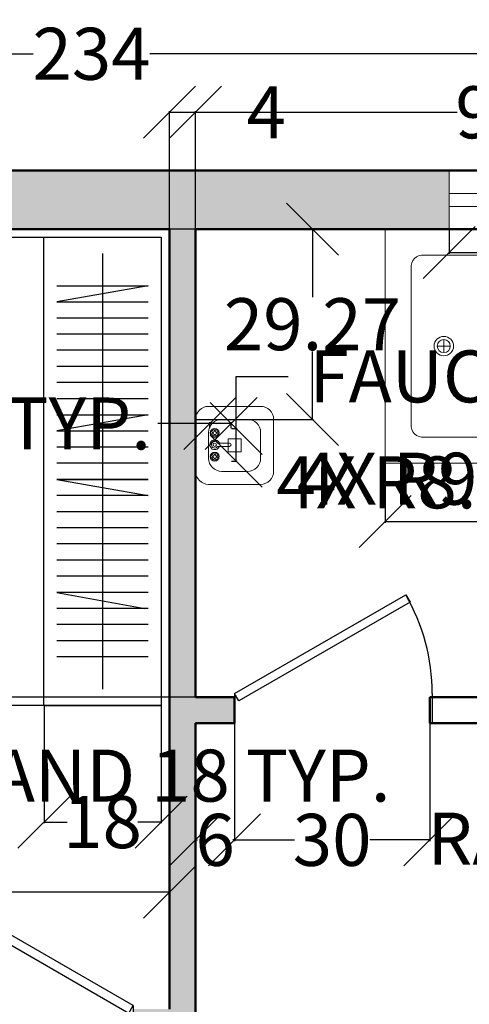
# Model space of a CAD drawing. Units: inches. Extents: x -87 to 308, y -349 to 42.
# Tile 5 of 6: x 119 to 188, y -110 to 42. Entities that reach past the tile are written whole.
import ezdxf

# ---------------------------------------------------------------- set-up
doc = ezdxf.new("R2010")
doc.units = ezdxf.units.IN
doc.header["$MEASUREMENT"] = 0
for name, color, linetype, lineweight in [('A-ANNO-DIMS', 2, 'Continuous', 18), ('A-DOOR', 3, 'Continuous', 25), ('A-FLOR-CASE', 9, 'Continuous', 25), ('A-FLOR-FIXT', 9, 'Continuous', 18), ('A-GLAZ', 4, 'Continuous', 18), ('A-WALL', 7, 'Continuous', 50), ('A-WALL-PATT', 251, 'Continuous', 13)]:
    doc.layers.add(name, color=color, linetype=linetype, lineweight=lineweight)
doc.styles.get("Standard").update_dxf_attribs({"font": 'arial.ttf'})
doc.dimstyles.get("Standard").update_dxf_attribs({"dimtxt": 8, "dimasz": 8, "dimexe": 0.18, "dimexo": 0.0625, "dimgap": 0.09, "dimtad": 0, "dimtih": 1, "dimtoh": 1, "dimdec": 0, "dimzin": 0, "dimdsep": 46, "dimlunit": 4, "dimtxsty": 'Standard', "dimblk": 'OBLIQUE', "dimcen": 0.09, "dimadec": 0, "dimazin": 0, "dimtfac": 1, "dimtdec": 0, "dimtofl": 0, "dimtmove": 0, "dimatfit": 3, "dimldrblk": 'OBLIQUE', "dimfxl": 1, "dimtolj": 1, "dimtzin": 0, "dimarcsym": 0})

# ---------------------------------------------------------------- blocks, each defined once
blk = doc.blocks.new('*U5')
for p, q in [((0, 0), (0, -6)), ((-40, 0), (-40, -6))]:
    blk.add_line(p, q)
blk.add_lwpolyline([(0, 0), (-34.64, 20), (-35.52, 18.48), (-0.88, -1.52)], close=True)
blk.add_arc((0, 0), 40, 150, 180)
blk = doc.blocks.new('*U4')
for p, q in [((0, 0), (0, -6)), ((40, 0), (40, -6))]:
    blk.add_line(p, q)
blk.add_lwpolyline([(0, 0), (34.64, 20), (35.52, 18.48), (0.87, -1.52)], close=True)
blk.add_arc((0, 0), 40, 0, 30)
blk = doc.blocks.new('Bath Tub - 26 x 60 in.')
for p, q in [((8, -18), (10, -18)), ((9, -17), (9, -19))]:
    blk.add_line(p, q)
blk.add_lwpolyline([(0, -36), (0, 0), (60, 0), (60, -36)], close=True)
for points in [[(6, -4), (42, -4)], [(4, -30), (4, -6)], [(42, -32), (6, -32)]]:
    blk.add_lwpolyline(points)
for radius in [1.5, 1]:
    blk.add_circle((9, -18), radius)
for centre, radius, start, end in [((5.75, -5.75), 1.77, 81.8699, 188.1301), ((42, -18), 14, 270, 90), ((5.75, -30.25), 1.77, 171.8699, 278.1301)]:
    blk.add_arc(centre, radius, start, end)
blk = doc.blocks.new('Faucet - Bathroom top')
for p, q in [((-4.107, 0.125), (-4.375, 0.125)), ((-3.75, 0.4788), (-3.75, 0.75)), ((-3.5, 0.482), (-3.5, 0.75)), ((-3.1461, 0.125), (-2.875, 0.125)), ((3.143, 0.125), (2.875, 0.125)), ((3.5, 0.4788), (3.5, 0.75)), ((3.75, 0.482), (3.75, 0.75)), ((4.1039, 0.125), (4.375, 0.125)), ((-4.1039, -0.125), (-4.375, -0.125)), ((-3.75, -0.4821), (-3.75, -0.75)), ((-3.5, -0.4789), (-3.5, -0.75)), ((-3.143, -0.125), (-2.875, -0.125)), ((-0.5, -0.8639), (-0.5, -4.5)), ((0.5, -4.5), (0.5, -0.8631)), ((3.1461, -0.125), (2.875, -0.125)), ((3.5, -0.4821), (3.5, -0.75)), ((3.75, -0.4789), (3.75, -0.75)), ((4.107, -0.125), (4.375, -0.125))]:
    blk.add_line(p, q)
for centre, radius in [((-3.625, 0), 1.375), ((-4.625, 0), 0.2795), ((-3.625, 0), 0.5), ((-3.625, 1), 0.2795), ((-2.625, 0), 0.2795), ((0, 0), 0.5), ((3.625, 0), 1.375), ((2.625, 0), 0.2795), ((3.625, 0), 0.5), ((3.625, 1), 0.2795), ((4.625, 0), 0.2795), ((-3.625, -1), 0.2795), ((3.625, -1), 0.2795)]:
    blk.add_circle(centre, radius)
for centre, radius, start, end in [((-3.625, 0), 1, 105.2407, 164.2093), ((-3.625, 0), 1, 16.44125, 74.07887), ((0, 0), 1.5, 289.6514, 250.3603), ((0, 0), 1, 300.3431, 239.7554), ((3.625, 0), 1, 106.12, 164.0884), ((3.625, 0), 1, 16.23422, 73.90469), ((-3.625, 0), 1, 196.2342, 253.9047), ((-3.625, 0), 1, 286.12, 344.0884), ((3.625, 0), 1, 196.4413, 254.0789), ((3.625, 0), 1, 285.2407, 344.2093), ((0, -4.5), 0.5, 180, 0)]:
    blk.add_arc(centre, radius, start, end)
blk = doc.blocks.new('WIN-24IN')
for p, q in [((0, 5.5), (24, 5.5)), ((0, 3.5), (24, 3.5))]:
    blk.add_line(p, q)
for points in [[(0, 0), (0, 9)], [(24, 9), (24, 0)]]:
    blk.add_lwpolyline(points)
blk = doc.blocks.new('LAVATORY-12IN')
for p, q in [((2, 12), (10, 12)), ((0, 2), (0, 10)), ((4, 10), (8, 10)), ((12, 10), (12, 2)), ((2, 4), (2, 8)), ((10, 8), (10, 4)), ((5, 7), (7, 7)), ((5, 5), (5, 7)), ((7, 7), (7, 5)), ((7, 5), (5, 5)), ((8, 2), (4, 2)), ((10, 0), (2, 0))]:
    blk.add_line(p, q)
for centre, start, end in [((2, 10), 90, 180), ((10, 10), 0, 90), ((4, 8), 90, 180), ((8, 8), 0, 90), ((4, 4), 180, 270), ((8, 4), 270, 0), ((2, 2), 180, 270), ((10, 2), 270, 0)]:
    blk.add_arc(centre, 2, start, end)
blk = doc.blocks.new('_Oblique')
at = {"color": 0, "linetype": 'ByBlock', "lineweight": -2}
blk.add_line((-0.5, -0.5), (0.5, 0.5), dxfattribs=at)
blk = doc.blocks.new('*D25')
at = {"layer": 'A-ANNO-DIMS', "color": 0, "lineweight": -2, "transparency": 16777216}
for p, q in [((184.75, 9.27), (184.75, 5.55)), ((208.75, 9.27), (208.75, 5.55)), ((184.75, 5.73), (208.75, 5.73)), ((208.75, 5.73), (216.75, 5.73))]:
    blk.add_line(p, q, dxfattribs=at)
at = {"layer": 'Defpoints', "color": 0, "transparency": 16777216}
for p in [(184.75, 9.33), (208.75, 9.33), (208.75, 5.73)]:
    blk.add_point(p, dxfattribs=at)
at = {"layer": 'A-ANNO-DIMS', "color": 0, "lineweight": -2, "transparency": 16777216, "xscale": 8, "yscale": 8, "zscale": 8, "rotation": 180}
blk.add_blockref('_Oblique', (184.75, 5.73), dxfattribs=at)
at = {"layer": 'A-ANNO-DIMS', "color": 0, "lineweight": -2, "transparency": 16777216, "xscale": 8, "yscale": 8, "zscale": 8}
blk.add_blockref('_Oblique', (208.75, 5.73), dxfattribs=at)
at = {"layer": 'A-ANNO-DIMS', "color": 0, "transparency": 16777216, "insert": (262.54, 5.73), "char_height": 8, "attachment_point": 5}
blk.add_mtext('\\A1;WINDOW 24 TYP.', dxfattribs=at)
blk = doc.blocks.new('*D31')
at = {"layer": 'A-ANNO-DIMS', "color": 0, "lineweight": -2, "transparency": 16777216}
for p, q in [((151.98, -21.33), (151.98, -13.33)), ((151.98, -13.33), (159.98, -13.33)), ((151.29, -21.33), (152.16, -21.33)), ((151.98, -26.36), (151.98, -21.33)), ((151.29, -26.36), (152.16, -26.36))]:
    blk.add_line(p, q, dxfattribs=at)
at = {"layer": 'Defpoints', "color": 0, "transparency": 16777216}
for p in [(151.23, -21.33), (151.98, -21.33), (151.23, -26.36)]:
    blk.add_point(p, dxfattribs=at)
at = {"layer": 'A-ANNO-DIMS', "color": 0, "lineweight": -2, "transparency": 16777216, "xscale": 8, "yscale": 8, "zscale": 8}
for p, rotation in [((151.98, -21.33), 90), ((151.98, -26.36), 270)]:
    blk.add_blockref('_Oblique', p, dxfattribs=dict(at, rotation=rotation))
at = {"layer": 'A-ANNO-DIMS', "color": 0, "transparency": 16777216, "insert": (200.11, -13.33), "char_height": 8, "attachment_point": 5}
blk.add_mtext('\\A1;FAUCET 5 TYP.', dxfattribs=at)
blk = doc.blocks.new('*D32')
at = {"layer": 'A-ANNO-DIMS', "color": 0, "lineweight": -2, "transparency": 16777216}
for p, q in [((147.96, -20.57), (139.96, -20.57)), ((147.96, -21.27), (147.96, -20.39)), ((151.23, -20.57), (147.96, -20.57)), ((151.23, -21.27), (151.23, -20.39))]:
    blk.add_line(p, q, dxfattribs=at)
at = {"layer": 'Defpoints', "color": 0, "transparency": 16777216}
for p in [(147.96, -20.57), (147.96, -21.33), (151.23, -21.33)]:
    blk.add_point(p, dxfattribs=at)
at = {"layer": 'A-ANNO-DIMS', "color": 0, "lineweight": -2, "transparency": 16777216, "xscale": 8, "yscale": 8, "zscale": 8, "rotation": 180}
blk.add_blockref('_Oblique', (147.96, -20.57), dxfattribs=at)
at = {"layer": 'A-ANNO-DIMS', "color": 0, "lineweight": -2, "transparency": 16777216, "xscale": 8, "yscale": 8, "zscale": 8}
blk.add_blockref('_Oblique', (151.23, -20.57), dxfattribs=at)
at = {"layer": 'A-ANNO-DIMS', "color": 0, "transparency": 16777216, "insert": (123.51, -20.57), "char_height": 8, "attachment_point": 5}
blk.add_mtext('\\A1;3 TYP.', dxfattribs=at)
blk = doc.blocks.new('*D37')
at = {"layer": 'A-ANNO-DIMS', "color": 0, "lineweight": -2, "transparency": 16777216}
for p, q in [((25.45, -77.37), (25.45, -74.56)), ((25.45, -74.74), (43.45, -74.74)), ((43.45, -77.37), (43.45, -74.56)), ((43.45, -74.74), (51.45, -74.74))]:
    blk.add_line(p, q, dxfattribs=at)
at = {"layer": 'Defpoints', "color": 0, "transparency": 16777216}
for p in [(43.45, -74.74), (25.45, -77.44), (43.45, -77.44)]:
    blk.add_point(p, dxfattribs=at)
at = {"layer": 'A-ANNO-DIMS', "color": 0, "lineweight": -2, "transparency": 16777216, "xscale": 8, "yscale": 8, "zscale": 8, "rotation": 180}
blk.add_blockref('_Oblique', (25.45, -74.74), dxfattribs=at)
at = {"layer": 'A-ANNO-DIMS', "color": 0, "lineweight": -2, "transparency": 16777216, "xscale": 8, "yscale": 8, "zscale": 8}
blk.add_blockref('_Oblique', (43.45, -74.74), dxfattribs=at)
at = {"layer": 'A-ANNO-DIMS', "color": 0, "transparency": 16777216, "insert": (115.81, -74.74), "char_height": 8, "attachment_point": 5}
blk.add_mtext('\\A1;R. NIGHTSTAND 18 TYP.', dxfattribs=at)
blk = doc.blocks.new('*D41')
at = {"layer": 'A-ANNO-DIMS', "color": 0, "lineweight": -2, "transparency": 16777216}
for p, q in [((210.82, -69.44), (206.2, -69.44)), ((206.38, -69.44), (206.38, -80.21)), ((206.38, -99.44), (206.38, -88.66)), ((210.82, -99.44), (206.2, -99.44))]:
    blk.add_line(p, q, dxfattribs=at)
at = {"layer": 'Defpoints', "color": 0, "transparency": 16777216}
for p in [(210.88, -69.44), (206.38, -99.44), (210.88, -99.44)]:
    blk.add_point(p, dxfattribs=at)
at = {"layer": 'A-ANNO-DIMS', "color": 0, "lineweight": -2, "transparency": 16777216, "xscale": 8, "yscale": 8, "zscale": 8}
for p, rotation in [((206.38, -69.44), 90), ((206.38, -99.44), 270)]:
    blk.add_blockref('_Oblique', p, dxfattribs=dict(at, rotation=rotation))
at = {"layer": 'A-ANNO-DIMS', "color": 0, "transparency": 16777216, "insert": (206.38, -84.44), "char_height": 8, "attachment_point": 5}
blk.add_mtext('\\A1;RANGE 30', dxfattribs=at)
blk = doc.blocks.new('*D45')
at = {"layer": 'A-ANNO-DIMS', "color": 0, "lineweight": -2, "transparency": 16777216}
for p, q in [((174.93, -26.73), (174.93, -35.85)), ((234.93, -26.73), (234.93, -35.85)), ((174.93, -35.67), (234.93, -35.67)), ((234.93, -35.67), (242.93, -35.67))]:
    blk.add_line(p, q, dxfattribs=at)
at = {"layer": 'Defpoints', "color": 0, "transparency": 16777216}
for p in [(174.93, -26.67), (234.93, -26.67), (234.93, -35.67)]:
    blk.add_point(p, dxfattribs=at)
at = {"layer": 'A-ANNO-DIMS', "color": 0, "lineweight": -2, "transparency": 16777216, "xscale": 8, "yscale": 8, "zscale": 8, "rotation": 180}
blk.add_blockref('_Oblique', (174.93, -35.67), dxfattribs=at)
at = {"layer": 'A-ANNO-DIMS', "color": 0, "lineweight": -2, "transparency": 16777216, "xscale": 8, "yscale": 8, "zscale": 8}
blk.add_blockref('_Oblique', (234.93, -35.67), dxfattribs=at)
at = {"layer": 'A-ANNO-DIMS', "color": 0, "transparency": 16777216, "insert": (276.19, -35.67), "char_height": 8, "attachment_point": 5}
blk.add_mtext('\\A1;BATHTUB 60', dxfattribs=at)
blk = doc.blocks.new('*D47')
at = {"layer": 'A-ANNO-DIMS', "color": 0, "lineweight": -2, "transparency": 16777216}
for p, q in [((12.76, 18.39), (12.76, 36.48)), ((246.76, 18.39), (246.76, 36.48)), ((12.76, 36.3), (120.78, 36.3)), ((246.76, 36.3), (138.74, 36.3))]:
    blk.add_line(p, q, dxfattribs=at)
at = {"layer": 'Defpoints', "color": 0, "transparency": 16777216}
for p in [(246.76, 36.3), (12.76, 18.33), (246.76, 18.33)]:
    blk.add_point(p, dxfattribs=at)
at = {"layer": 'A-ANNO-DIMS', "color": 0, "lineweight": -2, "transparency": 16777216, "xscale": 8, "yscale": 8, "zscale": 8, "rotation": 180}
blk.add_blockref('_Oblique', (12.76, 36.3), dxfattribs=at)
at = {"layer": 'A-ANNO-DIMS', "color": 0, "lineweight": -2, "transparency": 16777216, "xscale": 8, "yscale": 8, "zscale": 8}
blk.add_blockref('_Oblique', (246.76, 36.3), dxfattribs=at)
at = {"layer": 'A-ANNO-DIMS', "color": 0, "transparency": 16777216, "insert": (129.76, 36.3), "char_height": 8, "attachment_point": 5}
blk.add_mtext('\\A1;234', dxfattribs=at)
blk = doc.blocks.new('*D58')
at = {"layer": 'A-ANNO-DIMS', "color": 0, "lineweight": -2, "transparency": 16777216}
for p, q in [((21.76, -110.61), (21.76, -92.52)), ((21.76, -92.7), (73.23, -92.7)), ((141.76, -92.7), (90.3, -92.7)), ((141.76, -110.61), (141.76, -92.52))]:
    blk.add_line(p, q, dxfattribs=at)
at = {"layer": 'Defpoints', "color": 0, "transparency": 16777216}
for p in [(141.76, -92.7), (21.76, -110.67), (141.76, -110.67)]:
    blk.add_point(p, dxfattribs=at)
at = {"layer": 'A-ANNO-DIMS', "color": 0, "lineweight": -2, "transparency": 16777216, "xscale": 8, "yscale": 8, "zscale": 8, "rotation": 180}
blk.add_blockref('_Oblique', (21.76, -92.7), dxfattribs=at)
at = {"layer": 'A-ANNO-DIMS', "color": 0, "lineweight": -2, "transparency": 16777216, "xscale": 8, "yscale": 8, "zscale": 8}
blk.add_blockref('_Oblique', (141.76, -92.7), dxfattribs=at)
at = {"layer": 'A-ANNO-DIMS', "color": 0, "transparency": 16777216, "insert": (81.76, -92.7), "char_height": 8, "attachment_point": 5}
blk.add_mtext('\\A1;120', dxfattribs=at)
blk = doc.blocks.new('*D60')
at = {"layer": 'A-ANNO-DIMS', "color": 0, "lineweight": -2, "transparency": 16777216}
for p, q in [((145.7, 9.33), (-5.38, 9.33)), ((-5.2, 9.33), (-5.2, -22.56)), ((-5.2, -62.67), (-5.2, -30.77)), ((145.7, -62.67), (-5.38, -62.67))]:
    blk.add_line(p, q, dxfattribs=at)
at = {"layer": 'Defpoints', "color": 0, "transparency": 16777216}
for p in [(-5.2, 9.33), (145.76, 9.33), (145.76, -62.67)]:
    blk.add_point(p, dxfattribs=at)
at = {"layer": 'A-ANNO-DIMS', "color": 0, "lineweight": -2, "transparency": 16777216, "xscale": 8, "yscale": 8, "zscale": 8}
for p, rotation in [((-5.2, 9.33), 90), ((-5.2, -62.67), 270)]:
    blk.add_blockref('_Oblique', p, dxfattribs=dict(at, rotation=rotation))
at = {"layer": 'A-ANNO-DIMS', "color": 0, "transparency": 16777216, "insert": (-5.2, -26.67), "char_height": 8, "attachment_point": 5}
blk.add_mtext('\\A1;72', dxfattribs=at)
blk = doc.blocks.new('*D61')
at = {"layer": 'A-ANNO-DIMS', "color": 0, "lineweight": -2, "transparency": 16777216}
for p, q in [((145.76, 9.39), (145.76, 27.48)), ((145.76, 27.3), (185.98, 27.3)), ((237.76, 27.3), (197.54, 27.3)), ((237.76, 9.39), (237.76, 27.48))]:
    blk.add_line(p, q, dxfattribs=at)
at = {"layer": 'Defpoints', "color": 0, "transparency": 16777216}
for p in [(237.76, 27.3), (145.76, 9.33), (237.76, 9.33)]:
    blk.add_point(p, dxfattribs=at)
at = {"layer": 'A-ANNO-DIMS', "color": 0, "lineweight": -2, "transparency": 16777216, "xscale": 8, "yscale": 8, "zscale": 8, "rotation": 180}
blk.add_blockref('_Oblique', (145.76, 27.3), dxfattribs=at)
at = {"layer": 'A-ANNO-DIMS', "color": 0, "lineweight": -2, "transparency": 16777216, "xscale": 8, "yscale": 8, "zscale": 8}
blk.add_blockref('_Oblique', (237.76, 27.3), dxfattribs=at)
at = {"layer": 'A-ANNO-DIMS', "color": 0, "transparency": 16777216, "insert": (191.76, 27.3), "char_height": 8, "attachment_point": 5}
blk.add_mtext('\\A1;92', dxfattribs=at)
blk = doc.blocks.new('*D65')
at = {"layer": 'A-ANNO-DIMS', "color": 0, "lineweight": -2, "transparency": 16777216}
for p, q in [((141.76, 9.39), (141.76, 27.48)), ((141.76, 27.3), (145.76, 27.3)), ((145.76, 9.39), (145.76, 27.48)), ((145.76, 27.3), (153.76, 27.3))]:
    blk.add_line(p, q, dxfattribs=at)
at = {"layer": 'Defpoints', "color": 0, "transparency": 16777216}
for p in [(145.76, 27.3), (141.76, 9.33), (145.76, 9.33)]:
    blk.add_point(p, dxfattribs=at)
at = {"layer": 'A-ANNO-DIMS', "color": 0, "lineweight": -2, "transparency": 16777216, "xscale": 8, "yscale": 8, "zscale": 8, "rotation": 180}
blk.add_blockref('_Oblique', (141.76, 27.3), dxfattribs=at)
at = {"layer": 'A-ANNO-DIMS', "color": 0, "lineweight": -2, "transparency": 16777216, "xscale": 8, "yscale": 8, "zscale": 8}
blk.add_blockref('_Oblique', (145.76, 27.3), dxfattribs=at)
at = {"layer": 'A-ANNO-DIMS', "color": 0, "transparency": 16777216, "insert": (156.62, 27.3), "char_height": 8, "attachment_point": 5}
blk.add_mtext('\\A1;4', dxfattribs=at)
blk = doc.blocks.new('*D68')
at = {"layer": 'A-ANNO-DIMS', "color": 0, "lineweight": -2, "transparency": 16777216}
for p, q in [((145.76, -66.73), (145.76, -84.81)), ((151.76, -66.73), (151.76, -84.81)), ((145.76, -84.63), (146.03, -84.63)), ((151.76, -84.63), (151.49, -84.63))]:
    blk.add_line(p, q, dxfattribs=at)
at = {"layer": 'Defpoints', "color": 0, "transparency": 16777216}
for p in [(145.76, -66.67), (151.76, -66.67), (145.76, -84.63)]:
    blk.add_point(p, dxfattribs=at)
at = {"layer": 'A-ANNO-DIMS', "color": 0, "lineweight": -2, "transparency": 16777216, "xscale": 8, "yscale": 8, "zscale": 8, "rotation": 180.0000000000004}
blk.add_blockref('_Oblique', (145.76, -84.63), dxfattribs=at)
at = {"layer": 'A-ANNO-DIMS', "color": 0, "lineweight": -2, "transparency": 16777216, "xscale": 8, "yscale": 8, "zscale": 8}
blk.add_blockref('_Oblique', (151.76, -84.63), dxfattribs=at)
at = {"layer": 'A-ANNO-DIMS', "color": 0, "transparency": 16777216, "insert": (148.76, -84.63), "char_height": 8, "attachment_point": 5}
blk.add_mtext('\\A1;6', dxfattribs=at)
blk = doc.blocks.new('*D69')
at = {"layer": 'A-ANNO-DIMS', "color": 0, "lineweight": -2, "transparency": 16777216}
for p, q in [((151.76, -66.73), (151.76, -84.81)), ((181.76, -66.73), (181.76, -84.81)), ((151.76, -84.63), (160.96, -84.63)), ((181.76, -84.63), (172.57, -84.63))]:
    blk.add_line(p, q, dxfattribs=at)
at = {"layer": 'Defpoints', "color": 0, "transparency": 16777216}
for p in [(151.76, -66.67), (181.76, -66.67), (151.76, -84.63)]:
    blk.add_point(p, dxfattribs=at)
at = {"layer": 'A-ANNO-DIMS', "color": 0, "lineweight": -2, "transparency": 16777216, "xscale": 8, "yscale": 8, "zscale": 8, "rotation": 180.0000000000004}
blk.add_blockref('_Oblique', (151.76, -84.63), dxfattribs=at)
at = {"layer": 'A-ANNO-DIMS', "color": 0, "lineweight": -2, "transparency": 16777216, "xscale": 8, "yscale": 8, "zscale": 8}
blk.add_blockref('_Oblique', (181.76, -84.63), dxfattribs=at)
at = {"layer": 'A-ANNO-DIMS', "color": 0, "transparency": 16777216, "insert": (166.76, -84.63), "char_height": 8, "attachment_point": 5}
blk.add_mtext('\\A1;30', dxfattribs=at)
blk = doc.blocks.new('*D81')
at = {"layer": 'A-ANNO-DIMS', "color": 0, "lineweight": -2, "transparency": 16777216}
for p, q in [((122.45, -64), (122.45, -82.08)), ((140.45, -64), (140.45, -82.08)), ((122.45, -81.9), (125.99, -81.9)), ((140.45, -81.9), (136.9, -81.9))]:
    blk.add_line(p, q, dxfattribs=at)
at = {"layer": 'Defpoints', "color": 0, "transparency": 16777216}
for p in [(122.45, -63.94), (140.45, -63.94), (122.45, -81.9)]:
    blk.add_point(p, dxfattribs=at)
at = {"layer": 'A-ANNO-DIMS', "color": 0, "lineweight": -2, "transparency": 16777216, "xscale": 8, "yscale": 8, "zscale": 8, "rotation": 180}
blk.add_blockref('_Oblique', (122.45, -81.9), dxfattribs=at)
at = {"layer": 'A-ANNO-DIMS', "color": 0, "lineweight": -2, "transparency": 16777216, "xscale": 8, "yscale": 8, "zscale": 8}
blk.add_blockref('_Oblique', (140.45, -81.9), dxfattribs=at)
at = {"layer": 'A-ANNO-DIMS', "color": 0, "transparency": 16777216, "insert": (131.45, -81.9), "char_height": 8, "attachment_point": 5}
blk.add_mtext('\\A1;18', dxfattribs=at)
blk = doc.blocks.new('*D82')
at = {"layer": 'A-ANNO-DIMS', "color": 0, "lineweight": -2, "transparency": 16777216}
for p, q in [((122.38, 8.06), (104.3, 8.06)), ((104.48, 8.06), (104.48, -23.83)), ((104.48, -63.94), (104.48, -32.04)), ((122.38, -63.94), (104.3, -63.94))]:
    blk.add_line(p, q, dxfattribs=at)
at = {"layer": 'Defpoints', "color": 0, "transparency": 16777216}
for p in [(104.48, 8.06), (122.45, 8.06), (122.45, -63.94)]:
    blk.add_point(p, dxfattribs=at)
at = {"layer": 'A-ANNO-DIMS', "color": 0, "lineweight": -2, "transparency": 16777216, "xscale": 8, "yscale": 8, "zscale": 8}
for p, rotation in [((104.48, 8.06), 90), ((104.48, -63.94), 270)]:
    blk.add_blockref('_Oblique', p, dxfattribs=dict(at, rotation=rotation))
at = {"layer": 'A-ANNO-DIMS', "color": 0, "transparency": 16777216, "insert": (104.48, -27.94), "char_height": 8, "attachment_point": 5}
blk.add_mtext('\\A1;72', dxfattribs=at)
blk = doc.blocks.new('*D86')
at = {"layer": 'A-ANNO-DIMS', "color": 0, "lineweight": -2, "transparency": 16777216}
for p, q in [((145.83, 9.33), (163.91, 9.33)), ((163.73, 9.33), (163.73, -1.13)), ((163.73, -19.94), (163.73, -9.48)), ((145.83, -19.94), (163.91, -19.94))]:
    blk.add_line(p, q, dxfattribs=at)
at = {"layer": 'Defpoints', "color": 0, "transparency": 16777216}
for p in [(145.76, 9.33), (145.76, -19.94), (163.73, -19.94)]:
    blk.add_point(p, dxfattribs=at)
at = {"layer": 'A-ANNO-DIMS', "color": 0, "lineweight": -2, "transparency": 16777216, "xscale": 8, "yscale": 8, "zscale": 8}
for p, rotation in [((163.73, 9.33), 90), ((163.73, -19.94), 270)]:
    blk.add_blockref('_Oblique', p, dxfattribs=dict(at, rotation=rotation))
at = {"layer": 'A-ANNO-DIMS', "color": 0, "transparency": 16777216, "insert": (163.73, -5.3), "char_height": 8, "attachment_point": 5}
blk.add_mtext('\\A1;29.27', dxfattribs=at)
blk = doc.blocks.new('*D97')
at = {"layer": 'A-ANNO-DIMS', "color": 0, "lineweight": -2, "transparency": 16777216}
for p, q in [((205.86, -29.07), (213.86, -29.07)), ((213.86, -29.07), (217.93, -44.54)), ((220.23, -53.66), (220.41, -53.66)), ((220.32, -53.75), (220.32, -53.57))]:
    blk.add_line(p, q, dxfattribs=at)
at = {"layer": 'Defpoints', "color": 0, "transparency": 16777216}
for p in [(217.93, -44.54), (220.32, -53.66)]:
    blk.add_point(p, dxfattribs=at)
at = {"layer": 'A-ANNO-DIMS', "color": 0, "lineweight": -2, "transparency": 16777216, "xscale": 8, "yscale": 8, "zscale": 8, "rotation": 284.7189306886209}
blk.add_blockref('_Oblique', (217.93, -44.54), dxfattribs=at)
at = {"layer": 'A-ANNO-DIMS', "color": 0, "transparency": 16777216, "insert": (182.8, -29.07), "char_height": 8, "attachment_point": 5}
blk.add_mtext('\\A1;4X R9.43', dxfattribs=at)
blk = doc.blocks.new('*D98')
at = {"layer": 'A-ANNO-DIMS', "color": 0, "lineweight": -2, "transparency": 16777216}
for p, q in [((208.84, -29.63), (216.84, -29.63)), ((216.84, -29.63), (218.97, -45.49)), ((220.05, -54.19), (220.23, -54.19)), ((220.14, -54.28), (220.14, -54.1))]:
    blk.add_line(p, q, dxfattribs=at)
at = {"layer": 'Defpoints', "color": 0, "transparency": 16777216}
for p in [(218.97, -45.49), (220.14, -54.19)]:
    blk.add_point(p, dxfattribs=at)
at = {"layer": 'A-ANNO-DIMS', "color": 0, "lineweight": -2, "transparency": 16777216, "xscale": 8, "yscale": 8, "zscale": 8, "rotation": 277.6544285297157}
blk.add_blockref('_Oblique', (218.97, -45.49), dxfattribs=at)
at = {"layer": 'A-ANNO-DIMS', "color": 0, "transparency": 16777216, "insert": (182.66, -29.63), "char_height": 8, "attachment_point": 5}
blk.add_mtext('\\A1;4X R8.779', dxfattribs=at)

msp = doc.modelspace()

# ---------------------------------------------------------------- hatches: boundary and pattern name
at = {"layer": 'A-WALL-PATT'}
h = msp.add_hatch(color=256, dxfattribs=at)
h.dxf.hatch_style = 1
h.paths.add_polyline_path([(184.748, 18.332), (84.6671, 18.332), (84.6671, 9.332), (141.7637, 9.332), (141.7637, -110.668), (136.146, -110.668), (136.146, -114.668), (145.7637, -114.668), (145.7637, -66.668), (151.7637, -66.668), (151.7637, -62.668), (145.7637, -62.668), (145.7637, 9.332), (184.748, 9.332)])

# ---------------------------------------------------------------- linework, layer by layer
at = {"layer": 'A-FLOR-CASE'}
for p, q in [((131.4465, 5.5821), (131.4465, -61.4524)), ((138.4465, -4.3489), (124.4465, -4.3489)), ((138.4465, -6.8317), (124.4465, -6.8317)), ((138.4465, -9.3144), (124.4465, -9.3144)), ((138.4465, -11.7972), (124.4465, -11.7972)), ((138.4465, -14.2799), (124.4465, -14.2799)), ((138.4465, -16.7627), (124.4465, -16.7627)), ((138.4465, -24.211), (124.4465, -24.211)), ((138.4465, -26.6937), (124.4465, -26.6937)), ((138.4465, -34.142), (124.4465, -34.142)), ((138.4465, -36.6248), (124.4465, -36.6248)), ((138.4465, -39.1075), (124.4465, -39.1075)), ((138.4465, -41.5903), (124.4465, -41.5903)), ((138.4465, -44.073), (124.4465, -44.073)), ((138.4465, -49.0386), (124.4465, -49.0386)), ((138.4465, -51.5213), (124.4465, -51.5213)), ((138.4465, -54.0041), (124.4465, -54.0041)), ((138.4465, -56.4868), (124.4465, -56.4868))]:
    msp.add_line(p, q, dxfattribs=at)
for points in [[(122.4465, -63.9351), (122.4465, 8.0649), (140.4465, 8.0649), (140.4465, -63.9351), (122.4465, -63.9351), (140.4465, -63.9351)], [(124.4465, 0.6166), (138.4465, 0.6166), (124.4465, -1.8662), (138.4465, -1.8662)], [(124.4465, -19.2455), (138.4465, -19.2455), (124.4465, -21.7282), (138.4465, -21.7282)], [(124.4465, -29.1765), (138.4465, -29.1765), (124.4465, -29.1765), (138.4465, -31.6593), (124.4465, -31.6593)], [(138.4465, -46.5558), (124.4465, -46.5558), (137.9465, -49.0386)]]:
    msp.add_lwpolyline(points, dxfattribs=at)
at = {"layer": 'A-WALL'}
for p, q in [((21.7637, 9.332), (141.7637, 9.332)), ((141.7637, -110.668), (141.7637, 9.332)), ((145.7637, 9.332), (237.7637, 9.332)), ((145.7637, -62.668), (145.7637, 9.332)), ((145.7637, -62.668), (151.7637, -62.668)), ((151.7637, -62.668), (151.7637, -66.668)), ((181.7637, -62.668), (181.7637, -66.668)), ((181.7637, -62.668), (237.7637, -62.668)), ((145.7637, -114.668), (145.7637, -66.668)), ((145.7637, -66.668), (151.7637, -66.668)), ((181.7637, -66.668), (237.7637, -66.668))]:
    msp.add_line(p, q, dxfattribs=at)
msp.add_lwpolyline([(142.7127, -323.668), (12.7637, -323.668), (12.7637, 18.332), (246.7637, 18.332), (246.7637, -323.668), (172.7127, -323.668)], dxfattribs=at)

# ---------------------------------------------------------------- block references
at = {"layer": 'A-DOOR', "xscale": 0.7595575434647344, "yscale": 0.7595575434647344, "zscale": 0.7595575434647344}
for name, p in [('*U4', (151.7637, -62.1107)), ('*U5', (136.146, -110.1107))]:
    msp.add_blockref(name, p, dxfattribs=at)
at = {"layer": 'A-FLOR-FIXT'}
for name, p in [('Bath Tub - 26 x 60 in.', (174.9321, 9.332)), ('LAVATORY-12IN', (145.764, -29.935))]:
    msp.add_blockref(name, p, dxfattribs=at)
at = {"layer": 'A-FLOR-FIXT', "xscale": 0.5034362513714087, "yscale": 0.5034362513714087, "zscale": 0.5034362513714087, "rotation": 90}
msp.add_blockref('Faucet - Bathroom top', (148.7107, -23.847), dxfattribs=at)
at = {"layer": 'A-GLAZ'}
msp.add_blockref('WIN-24IN', (184.748, 9.332), dxfattribs=at)

# ---------------------------------------------------------------- dimensions: what is measured, and where the dimension line sits
at = {"layer": 'A-ANNO-DIMS'}
for base, p1, p2, picture, middle in [((246.7637, 36.2965), (12.7637, 18.332), (246.7637, 18.332), '*D47', (129.7637, 36.2965)), ((145.7637, 27.2965), (141.7637, 9.332), (145.7637, 9.332), '*D65', (156.6204, 27.2965)), ((237.7637, 27.2965), (145.7637, 9.332), (237.7637, 9.332), '*D61', (191.7637, 27.2965)), ((141.7637, -92.7035), (21.7637, -110.668), (141.7637, -110.668), '*D58', (81.7637, -92.7035))]:
    dim = msp.add_linear_dim(base=base, p1=p1, p2=p2, dimstyle='Standard', override={"dimdec": 0, "dimlfac": 1, "dimrnd": 0, "dimzin": 0, "dimdsep": 46, "dimlunit": 2}, dxfattribs=at)
    dim.commit()
    dim.dimension.update_dxf_attribs({"geometry": picture, "text_midpoint": middle})
for base, p1, p2, text, picture, middle in [((208.748, 5.732), (184.748, 9.332), (208.748, 9.332), 'WINDOW <> TYP.', '*D25', (262.5433, 5.732)), ((234.9321, -35.668), (174.9321, -26.668), (234.9321, -26.668), 'BATHTUB <>', '*D45', (276.1926, -35.668)), ((43.4465, -74.7351), (25.4465, -77.4351), (43.4465, -77.4351), 'R. NIGHTSTAND <> TYP.', '*D37', (115.8148, -74.7351))]:
    dim = msp.add_linear_dim(base=base, p1=p1, p2=p2, text=text, dimstyle='Standard', override={"dimdec": 0, "dimlfac": 1, "dimrnd": 0, "dimzin": 0, "dimdsep": 46, "dimlunit": 2}, dxfattribs=at)
    dim.commit()
    dim.dimension.update_dxf_attribs({"geometry": picture, "text_midpoint": middle})
for base, p1, p2, angle, override, picture, middle in [((-5.2008, 9.332), (145.7637, -62.668), (145.7637, 9.332), 90, {"dimdec": 0, "dimlfac": 1, "dimrnd": 0, "dimzin": 0, "dimdsep": 46, "dimlunit": 2}, '*D60', (-5.2008, -26.668)), ((163.7282, -19.9351), (145.7637, 9.332), (145.7637, -19.9351), 270, {"dimdec": 2, "dimlfac": 1, "dimrnd": 0, "dimzin": 0, "dimdsep": 46, "dimlunit": 2}, '*D86', (163.7282, -5.3016)), ((104.482, 8.0649), (122.4465, -63.9351), (122.4465, 8.0649), 90, {"dimdec": 0, "dimlfac": 1, "dimrnd": 0, "dimzin": 0, "dimdsep": 46, "dimlunit": 2}, '*D82', (104.482, -27.9351)), ((122.4465, -81.8996), (140.4465, -63.9351), (122.4465, -63.9351), 180, {"dimdec": 0, "dimlfac": 1, "dimrnd": 0, "dimzin": 0, "dimdsep": 46, "dimlunit": 2}, '*D81', (131.4465, -81.8996)), ((145.7637, -84.6325), (151.7637, -66.668), (145.7637, -66.668), 180, {"dimdec": 0, "dimlfac": 1, "dimrnd": 0, "dimzin": 0, "dimdsep": 46, "dimlunit": 2}, '*D68', (148.7637, -84.6325)), ((151.7637, -84.6325), (181.7637, -66.668), (151.7637, -66.668), 180, {"dimdec": 0, "dimlfac": 1, "dimrnd": 0, "dimzin": 0, "dimdsep": 46, "dimlunit": 2}, '*D69', (166.7637, -84.6325))]:
    dim = msp.add_linear_dim(base=base, p1=p1, p2=p2, angle=angle, dimstyle='Standard', override=override, dxfattribs=at)
    dim.commit()
    dim.dimension.update_dxf_attribs({"geometry": picture, "text_midpoint": middle})
for base, p1, p2, angle, text, picture, middle in [((151.983, -21.3298), (151.2279, -26.3642), (151.2279, -21.3298), 90, 'FAUCET <> TYP.', '*D31', (200.114, -13.3298)), ((147.9555, -20.5747), (151.2279, -21.3298), (147.9555, -21.3298), 180, '<> TYP.', '*D32', (123.5054, -20.5747)), ((206.3805, -99.4351), (210.8805, -69.4351), (210.8805, -99.4351), 270, 'RANGE <>', '*D41', (206.3805, -84.4351))]:
    dim = msp.add_linear_dim(base=base, p1=p1, p2=p2, angle=angle, text=text, dimstyle='Standard', override={"dimdec": 0, "dimlfac": 1, "dimrnd": 0, "dimzin": 0, "dimdsep": 46, "dimlunit": 2}, dxfattribs=at)
    dim.commit()
    dim.dimension.update_dxf_attribs({"geometry": picture, "text_midpoint": middle})
for center, mpoint, override, picture, middle in [((220.1403, -54.1895), (218.971, -45.4891), {"dimdec": 3, "dimlfac": 1, "dimrnd": 0, "dimzin": 0, "dimdsep": 46, "dimlunit": 2}, '*D98', (182.6598, -29.6317)), ((220.3239, -53.6623), (217.9281, -44.5423), {"dimdec": 2, "dimlfac": 1, "dimrnd": 0, "dimzin": 0, "dimdsep": 46, "dimlunit": 2}, '*D97', (182.7988, -29.0674))]:
    dim = msp.add_radius_dim(center=center, mpoint=mpoint, text='4X <>', dimstyle='Standard', override=override, dxfattribs=at)
    dim.commit()
    dim.dimension.update_dxf_attribs({"geometry": picture, "text_midpoint": middle})

doc.saveas('drawing.dxf')
